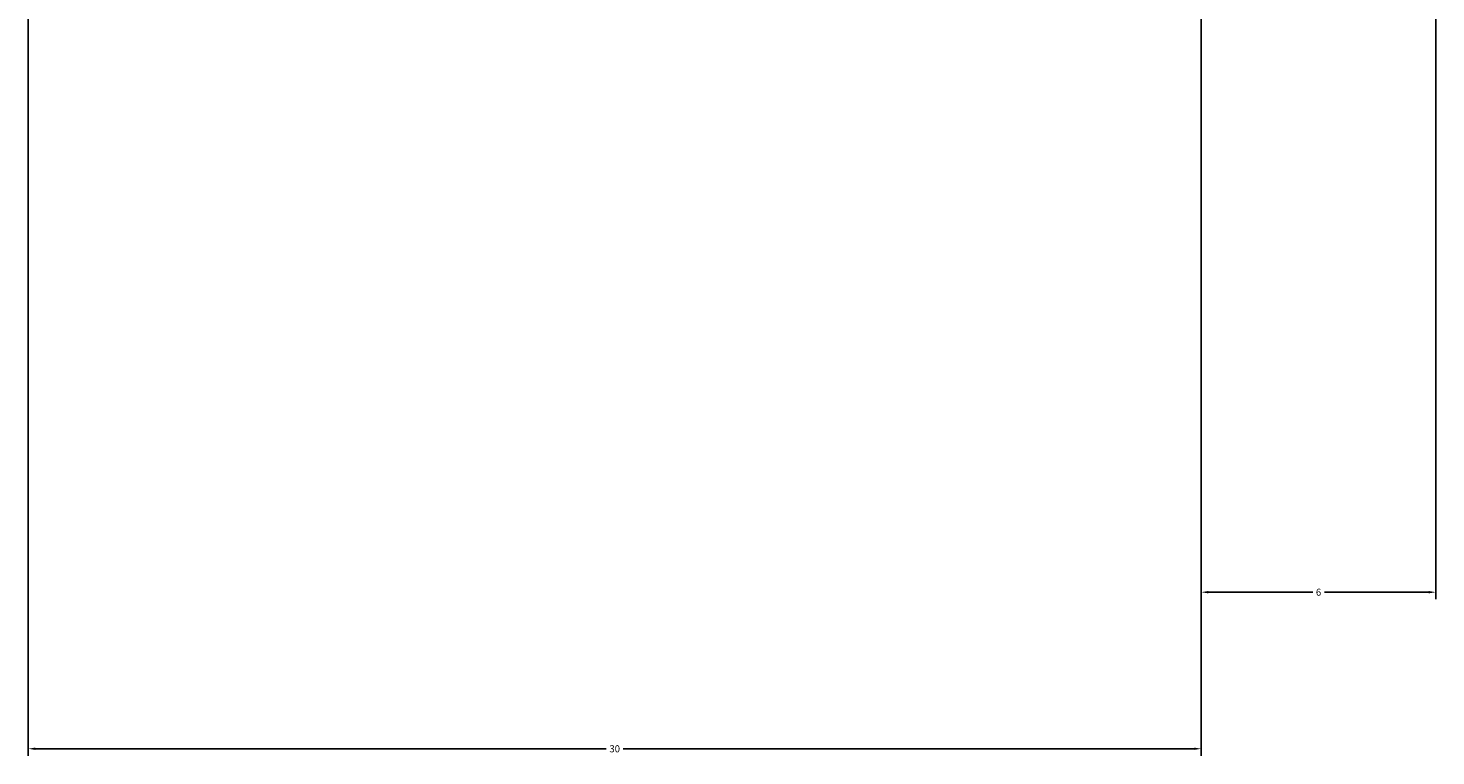
# Model space of a CAD drawing. Units: inches. Extents: x 2307 to 2544, y 2171 to 2540.
# Tile 19 of 52: x 2416 to 2452, y 2368 to 2387. Entities that reach past the tile are written whole.
import ezdxf

# ---------------------------------------------------------------- set-up
doc = ezdxf.new("R2010")
doc.units = ezdxf.units.IN
doc.layers.add('A-ANNO-DIMS', color=2, linetype='Continuous', lineweight=18)
doc.styles.get("Standard").update_dxf_attribs({"font": 'arial.ttf'})
doc.dimstyles.get("Standard").update_dxf_attribs({"dimtxt": 0.18, "dimasz": 0.18, "dimexe": 0.18, "dimexo": 0.0625, "dimgap": 0.09, "dimtad": 0, "dimtih": 1, "dimtoh": 1, "dimdec": 4, "dimzin": 0, "dimdsep": 46, "dimtxsty": 'Standard', "dimcen": 0.09, "dimadec": 0, "dimazin": 0, "dimtfac": 1, "dimtdec": 4, "dimtofl": 0, "dimtmove": 0, "dimatfit": 3, "dimfxl": 1, "dimtolj": 1, "dimtzin": 0, "dimarcsym": 0})

# ---------------------------------------------------------------- blocks, each defined once
blk = doc.blocks.new('*D51')
at = {"layer": 'A-ANNO-DIMS', "color": 0, "lineweight": -2, "transparency": 16777216}
for p, q in [((2415.696, 2387.447), (2415.696, 2368.18)), ((2445.696, 2387.447), (2445.696, 2368.18)), ((2415.876, 2368.36), (2430.477, 2368.36)), ((2445.516, 2368.36), (2430.914, 2368.36))]:
    blk.add_line(p, q, dxfattribs=at)
at = {"layer": 'A-ANNO-DIMS', "color": 0, "transparency": 16777216}
for points in [[(2415.876, 2368.39), (2415.876, 2368.33), (2415.696, 2368.36)], [(2445.516, 2368.39), (2445.516, 2368.33), (2445.696, 2368.36)]]:
    blk.add_solid(points, dxfattribs=at)
at = {"layer": 'Defpoints', "color": 0, "transparency": 16777216}
for p in [(2415.696, 2387.51), (2445.696, 2387.51), (2415.696, 2368.36)]:
    blk.add_point(p, dxfattribs=at)
at = {"layer": 'A-ANNO-DIMS', "color": 0, "transparency": 16777216, "insert": (2430.696, 2368.36), "char_height": 0.18, "attachment_point": 5}
blk.add_mtext('\\A1;30', dxfattribs=at)
blk = doc.blocks.new('*D52')
at = {"layer": 'A-ANNO-DIMS', "color": 0, "lineweight": -2, "transparency": 16777216}
for p, q in [((2445.696, 2391.447), (2445.696, 2372.18)), ((2451.696, 2391.447), (2451.696, 2372.18)), ((2445.876, 2372.36), (2448.546, 2372.36)), ((2451.516, 2372.36), (2448.845, 2372.36))]:
    blk.add_line(p, q, dxfattribs=at)
at = {"layer": 'A-ANNO-DIMS', "color": 0, "transparency": 16777216}
for points in [[(2445.876, 2372.39), (2445.876, 2372.33), (2445.696, 2372.36)], [(2451.516, 2372.39), (2451.516, 2372.33), (2451.696, 2372.36)]]:
    blk.add_solid(points, dxfattribs=at)
at = {"layer": 'Defpoints', "color": 0, "transparency": 16777216}
for p in [(2445.696, 2391.51), (2451.696, 2391.51), (2445.696, 2372.36)]:
    blk.add_point(p, dxfattribs=at)
at = {"layer": 'A-ANNO-DIMS', "color": 0, "transparency": 16777216, "insert": (2448.696, 2372.36), "char_height": 0.18, "attachment_point": 5}
blk.add_mtext('\\A1;6', dxfattribs=at)

msp = doc.modelspace()

# ---------------------------------------------------------------- dimensions: what is measured, and where the dimension line sits
at = {"layer": 'A-ANNO-DIMS'}
for base, p1, p2, picture, middle in [((2445.6958, 2372.3596), (2451.6958, 2391.5096), (2445.6958, 2391.5096), '*D52', (2448.6958, 2372.3596)), ((2415.6958, 2368.3596), (2445.6958, 2387.5096), (2415.6958, 2387.5096), '*D51', (2430.6958, 2368.3596))]:
    dim = msp.add_linear_dim(base=base, p1=p1, p2=p2, angle=180, dimstyle='Standard', override={"dimdec": 0, "dimlfac": 1, "dimrnd": 0, "dimzin": 0, "dimdsep": 46, "dimlunit": 2}, dxfattribs=at)
    dim.commit()
    dim.dimension.update_dxf_attribs({"geometry": picture, "text_midpoint": middle})

doc.saveas('drawing.dxf')
